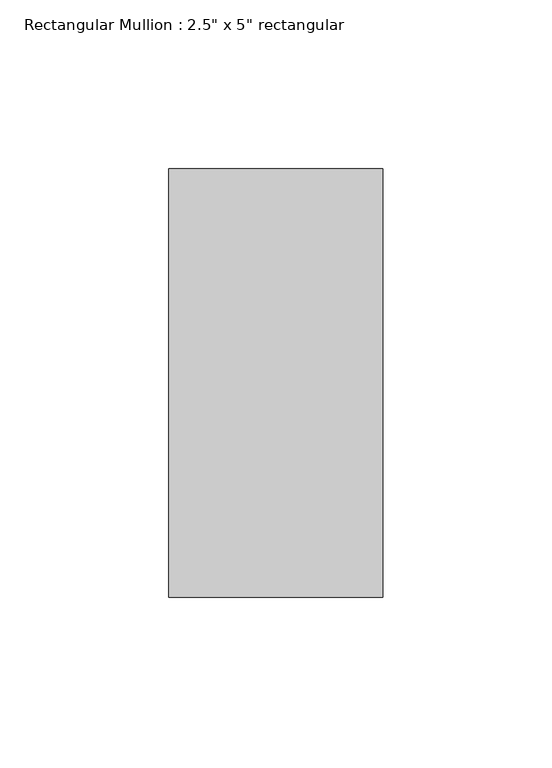
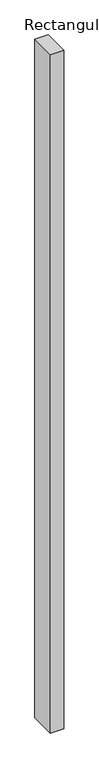
"""IFC4 building model written with IfcOpenShell, lengths in millimetres: member geometry."""

from ifc_helpers import new_model, si_unit, frame, origin, place, context, project, spatial, polyline, outline, extrude, source, transform, mapped, element, save


def member_78a27e2d(model_context):
    return source(origin(), model_context, "Body", "SweptSolid", [
        extrude(outline(polyline([(0.0, 63.5), (0.0, -63.5), (-63.5, -63.5), (-63.5, 63.5), (0.0, 63.5)])), frame((0.0, 0.0, -3400.1006278), z_axis=(0.0, 0.0, 1.0), x_axis=(1.0, 0.0, 0.0)), (0.0, 0.0, 1.0), 3400.1006278),
    ])


if __name__ == "__main__":
    model = new_model("IFC4")
    model_context = context("Model", 3, world=origin())
    ifc_project = project(units=[si_unit("LENGTHUNIT", "METRE", prefix="MILLI")], contexts=[model_context])
    site = spatial("IfcSite", under=ifc_project)
    building = spatial("IfcBuilding", under=site)
    placement = place(None, origin())
    member_shape = member_78a27e2d(model_context)
    element("IfcMember", 1, ObjectType="Rectangular Mullion : 2.5\" x 5\" rectangular", at=placement, inside=building, context=model_context, shape_type="MappedRepresentation", body=[
        mapped(member_shape, transform((0.0, 0.0, 0.0), x_axis=(1.0, 0.0, 0.0), y_axis=(0.0, 1.0, 0.0), z_axis=(0.0, 0.0, 1.0))),
    ])
    save(model, "model.ifc")

# Revit data of these elements
# Type "Rectangular Mullion : 2.5\" x 5\" rectangular"
#   built-in parameter 1007304 = 0.416667 (stored number, unit not read)
#   built-in parameter 1007301 = 0.104167 (stored number, unit not read)
#   built-in parameter 1007300 = 0.104167 (stored number, unit not read)
# Element 1 (IfcMember, "Rectangular Mullion : 2.5\" x 5\" rectangular")
#   Materials on its faces: "Iron, Ductile"
# Materials
#   "Iron, Ductile": class "Metal", colour RGB 0 0 0, transparency 0, Description = "Ductile cast iron", Cost = 0
